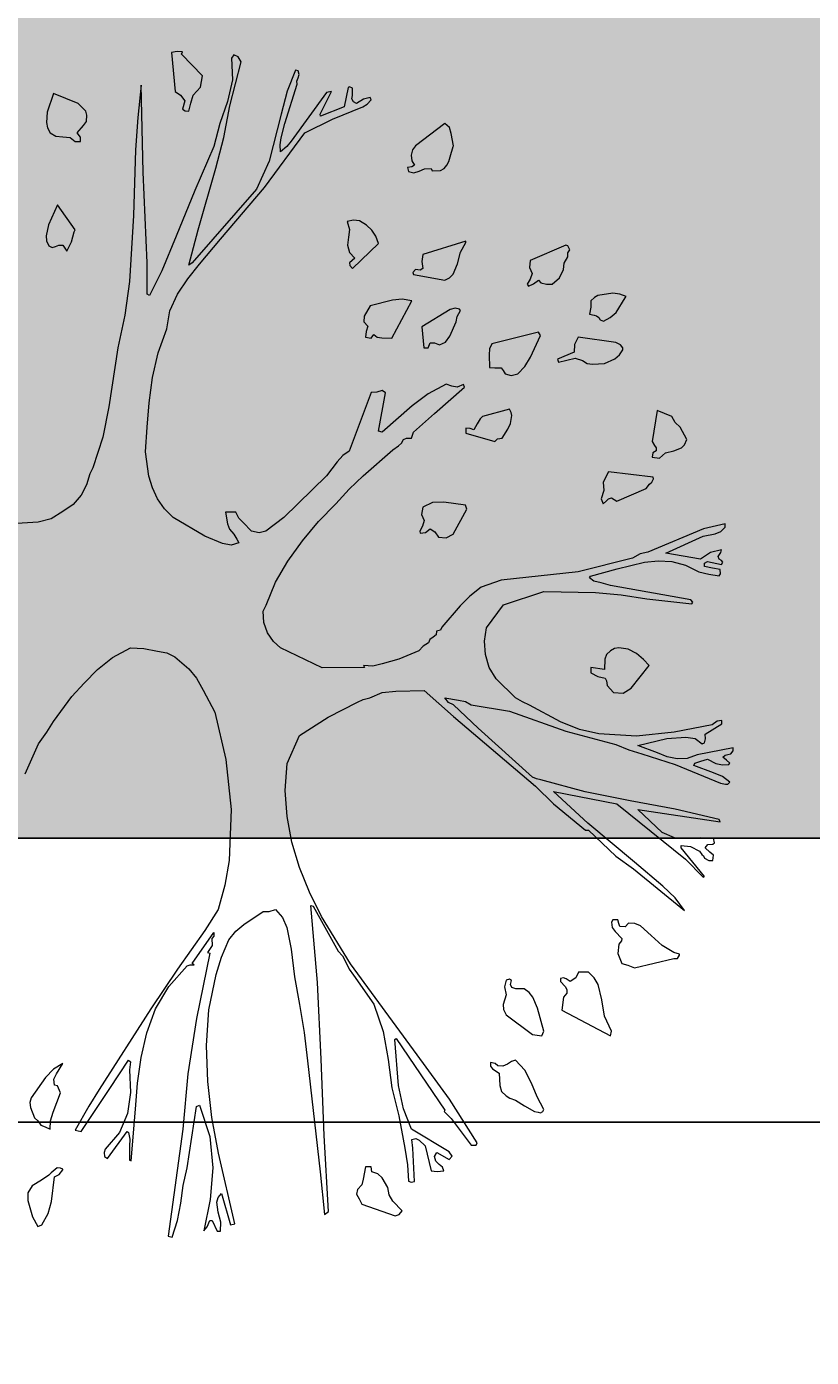
# Model space of a CAD drawing. Units: inches. Extents: x 84 to 1044, y -280 to 906.
# Tile 26 of 105: x 739 to 764, y -129 to -87. Entities that reach past the tile are written whole.
import ezdxf

# ---------------------------------------------------------------- set-up
doc = ezdxf.new("R2010")
doc.units = ezdxf.units.IN
for name, color, linetype, lineweight in [('A-ANNO-DIMS', 2, 'Continuous', 18), ('C-PROP', 7, 'Continuous', 25), ('L-PLNT', 114, 'Continuous', 15)]:
    doc.layers.add(name, color=color, linetype=linetype, lineweight=lineweight)
doc.layers.add('L-PLNT-PATT', color=9, linetype='Continuous', lineweight=9, true_color=0xafd9aa)
doc.styles.get("Standard").update_dxf_attribs({"font": 'arial.ttf'})
doc.dimstyles.get("Standard").update_dxf_attribs({"dimtxt": 0.18, "dimasz": 0.18, "dimexe": 0.18, "dimexo": 0.0625, "dimgap": 0.09, "dimtad": 0, "dimtih": 1, "dimtoh": 1, "dimdec": 4, "dimzin": 0, "dimdsep": 46, "dimtxsty": 'Standard', "dimcen": 0.09, "dimadec": 0, "dimazin": 0, "dimtfac": 1, "dimtdec": 4, "dimtofl": 0, "dimtmove": 0, "dimatfit": 3, "dimfxl": 1, "dimtolj": 1, "dimtzin": 0, "dimarcsym": 0})

# ---------------------------------------------------------------- blocks, each defined once
blk = doc.blocks.new('A$C37E508DF')
for p, q in [((0.7083, 1.5239), (0.7152, 1.5244)), ((0.7096, 1.5209), (0.7083, 1.5239)), ((0.7152, 1.5244), (0.7225, 1.5231)), ((0.7225, 1.5231), (0.7174, 1.4729)), ((0.6329, 1.5111), (0.6367, 1.5175)), ((0.6475, 1.4545), (0.6329, 1.5111)), ((0.6367, 1.5175), (0.6423, 1.5201)), ((0.6423, 1.5201), (0.6453, 1.5158)), ((0.6453, 1.5158), (0.644, 1.4879)), ((0.6826, 1.493), (0.7096, 1.5209)), ((0.5583, 1.4948), (0.5596, 1.4995)), ((0.5596, 1.4905), (0.5583, 1.4948)), ((0.5596, 1.4995), (0.563, 1.5003)), ((0.5613, 1.4862), (0.5596, 1.4905)), ((0.563, 1.5003), (0.5737, 1.4733)), ((0.6852, 1.4785), (0.6826, 1.493)), ((0.4897, 1.4772), (0.4935, 1.4789)), ((0.4897, 1.4678), (0.4897, 1.4772)), ((0.4935, 1.4789), (0.4952, 1.478)), ((0.4952, 1.478), (0.5004, 1.4532)), ((0.5313, 1.4437), (0.5167, 1.4729)), ((0.5167, 1.4729), (0.5231, 1.4716)), ((0.5231, 1.4716), (0.5686, 1.409)), ((0.5608, 1.4823), (0.5613, 1.4862)), ((0.5767, 1.4317), (0.5608, 1.4823)), ((0.5737, 1.4733), (0.5814, 1.4437)), ((0.644, 1.4879), (0.6505, 1.46)), ((0.6946, 1.4682), (0.6852, 1.4785)), ((0.7174, 1.4729), (0.7109, 1.4682)), ((0.7589, 1.3691), (0.7615, 1.481)), ((0.7615, 1.481), (0.7658, 1.4395)), ((0.4657, 1.4622), (0.4669, 1.4652)), ((0.4708, 1.4566), (0.4657, 1.4622)), ((0.4669, 1.4652), (0.4755, 1.463)), ((0.4764, 1.4532), (0.4708, 1.4566)), ((0.4755, 1.463), (0.4845, 1.4575)), ((0.4845, 1.4575), (0.4884, 1.4596)), ((0.4884, 1.4596), (0.4905, 1.4635)), ((0.4905, 1.4635), (0.4897, 1.4678)), ((0.6552, 1.4137), (0.6475, 1.4545)), ((0.6505, 1.46), (0.6603, 1.4317)), ((0.6976, 1.4579), (0.6946, 1.4682)), ((0.7002, 1.4476), (0.6976, 1.4579)), ((0.7109, 1.4682), (0.7053, 1.4609)), ((0.7053, 1.4609), (0.7083, 1.4502)), ((0.8357, 1.451), (0.8421, 1.4575)), ((0.8421, 1.4575), (0.8739, 1.4703)), ((0.8739, 1.4703), (0.882, 1.4463)), ((0.5154, 1.4373), (0.4764, 1.4532)), ((0.5004, 1.4532), (0.5308, 1.4412)), ((0.551, 1.4197), (0.5154, 1.4373)), ((0.5308, 1.4412), (0.5313, 1.4437)), ((0.5814, 1.4437), (0.5969, 1.3833)), ((0.7049, 1.448), (0.7002, 1.4476)), ((0.7083, 1.4502), (0.7049, 1.448)), ((0.7658, 1.4395), (0.7684, 1.3979)), ((0.831, 1.4424), (0.8323, 1.4476)), ((0.8318, 1.4343), (0.831, 1.4424)), ((0.8323, 1.4476), (0.8357, 1.451)), ((0.882, 1.4463), (0.8829, 1.433)), ((0.3628, 1.4189), (0.3649, 1.4266)), ((0.3649, 1.4266), (0.3709, 1.4317)), ((0.3709, 1.4317), (0.4086, 1.403)), ((0.5814, 1.4133), (0.5767, 1.4317)), ((0.6603, 1.4317), (0.668, 1.4021)), ((0.8353, 1.4292), (0.8318, 1.4343)), ((0.8434, 1.4197), (0.8353, 1.4292)), ((0.8816, 1.4262), (0.8781, 1.4197)), ((0.8829, 1.433), (0.8816, 1.4262)), ((0.3598, 1.403), (0.3628, 1.4189)), ((0.3602, 1.4021), (0.3598, 1.403)), ((0.4086, 1.403), (0.4125, 1.3979)), ((0.6029, 1.3494), (0.551, 1.4197)), ((0.5686, 1.409), (0.5741, 1.4021)), ((0.5827, 1.4043), (0.5814, 1.4133)), ((0.5823, 1.3953), (0.5827, 1.4043)), ((0.6655, 1.3743), (0.6552, 1.4137)), ((0.8391, 1.4141), (0.8434, 1.4197)), ((0.8395, 1.4086), (0.8391, 1.4141)), ((0.846, 1.4086), (0.8395, 1.4086)), ((0.8528, 1.4137), (0.846, 1.4086)), ((0.8619, 1.4146), (0.8528, 1.4137)), ((0.8709, 1.4154), (0.8619, 1.4146)), ((0.8781, 1.4197), (0.8709, 1.4154)), ((0.364, 1.3888), (0.3602, 1.4021)), ((0.3657, 1.3828), (0.364, 1.3888)), ((0.4125, 1.3979), (0.4142, 1.391)), ((0.4142, 1.391), (0.4134, 1.3837)), ((0.5741, 1.4021), (0.5823, 1.3953)), ((0.668, 1.4021), (0.6925, 1.3455)), ((0.7684, 1.3979), (0.771, 1.3134)), ((0.3683, 1.3781), (0.3657, 1.3828)), ((0.3718, 1.3738), (0.3683, 1.3781)), ((0.3765, 1.3713), (0.3718, 1.3738)), ((0.3872, 1.3708), (0.3765, 1.3713)), ((0.3885, 1.3738), (0.3872, 1.3708)), ((0.3971, 1.3734), (0.3885, 1.3738)), ((0.4039, 1.3704), (0.3971, 1.3734)), ((0.4108, 1.3683), (0.4039, 1.3704)), ((0.4134, 1.3837), (0.4099, 1.3781)), ((0.4099, 1.3781), (0.4134, 1.376)), ((0.4176, 1.37), (0.4108, 1.3683)), ((0.4134, 1.376), (0.4189, 1.3751)), ((0.4189, 1.3751), (0.4176, 1.37)), ((0.5969, 1.3833), (0.6132, 1.3472)), ((0.6882, 1.2949), (0.6655, 1.3743)), ((0.7538, 1.2529), (0.7589, 1.3691)), ((0.6595, 1.2829), (0.6029, 1.3494)), ((0.6132, 1.3472), (0.6959, 1.2529)), ((0.6925, 1.3455), (0.7161, 1.2868)), ((0.846, 1.2949), (0.8687, 1.3271)), ((0.8687, 1.3271), (0.8803, 1.3014)), ((0.4648, 1.2945), (0.4717, 1.3009)), ((0.4717, 1.3009), (0.4807, 1.3065)), ((0.4807, 1.3065), (0.4884, 1.3074)), ((0.4884, 1.3074), (0.4965, 1.3057)), ((0.4965, 1.3057), (0.4935, 1.2954)), ((0.771, 1.3134), (0.7761, 1.2285)), ((0.8803, 1.3014), (0.8833, 1.2872)), ((0.4562, 1.2774), (0.4597, 1.2868)), ((0.4597, 1.2868), (0.4648, 1.2945)), ((0.4935, 1.2954), (0.4948, 1.2855)), ((0.4948, 1.2855), (0.4961, 1.2756)), ((0.7002, 1.2495), (0.6882, 1.2949)), ((0.7161, 1.2868), (0.7349, 1.2422)), ((0.8473, 1.2924), (0.846, 1.2949)), ((0.8507, 1.2795), (0.8473, 1.2924)), ((0.8833, 1.2872), (0.8829, 1.2808)), ((0.2101, 1.2696), (0.2127, 1.2744)), ((0.2127, 1.2654), (0.2101, 1.2696)), ((0.2127, 1.2744), (0.2152, 1.2752)), ((0.2152, 1.2752), (0.2611, 1.2559)), ((0.3439, 1.2804), (0.3992, 1.2636)), ((0.3439, 1.2787), (0.3439, 1.2804)), ((0.3507, 1.2662), (0.3439, 1.2787)), ((0.3546, 1.2516), (0.3507, 1.2662)), ((0.4897, 1.2452), (0.4562, 1.2774)), ((0.4961, 1.2756), (0.4935, 1.2658)), ((0.6865, 1.2508), (0.6595, 1.2829)), ((0.8567, 1.2679), (0.8507, 1.2795)), ((0.8619, 1.2752), (0.8567, 1.2679)), ((0.867, 1.2752), (0.8619, 1.2752)), ((0.8713, 1.2739), (0.867, 1.2752)), ((0.8756, 1.2726), (0.8713, 1.2739)), ((0.8799, 1.2744), (0.8756, 1.2726)), ((0.8829, 1.2808), (0.8799, 1.2744)), ((0.2127, 1.2602), (0.2127, 1.2654)), ((0.2174, 1.2521), (0.2127, 1.2602)), ((0.2182, 1.2443), (0.2174, 1.2521)), ((0.2611, 1.2559), (0.262, 1.2465)), ((0.3602, 1.2383), (0.3546, 1.2516)), ((0.3992, 1.2636), (0.4005, 1.2546)), ((0.4005, 1.2546), (0.3992, 1.2452)), ((0.4935, 1.2658), (0.4867, 1.2589)), ((0.4867, 1.2589), (0.4935, 1.2529)), ((0.4931, 1.2491), (0.4897, 1.2452)), ((0.4935, 1.2529), (0.4931, 1.2491)), ((0.7015, 1.2323), (0.6865, 1.2508)), ((0.6959, 1.2529), (0.7002, 1.2495)), ((0.7538, 1.2122), (0.7538, 1.2529)), ((0.2234, 1.2336), (0.2182, 1.2443)), ((0.2328, 1.2251), (0.2234, 1.2336)), ((0.262, 1.2465), (0.2586, 1.2388)), ((0.2586, 1.2388), (0.2611, 1.2319)), ((0.2611, 1.2319), (0.265, 1.2251)), ((0.3649, 1.2336), (0.3602, 1.2383)), ((0.3709, 1.2306), (0.3649, 1.2336)), ((0.4112, 1.2375), (0.3709, 1.2306)), ((0.3992, 1.2452), (0.4026, 1.2431)), ((0.4026, 1.2431), (0.4086, 1.2443)), ((0.4086, 1.2443), (0.4121, 1.2401)), ((0.4121, 1.2401), (0.4112, 1.2375)), ((0.7148, 1.2126), (0.7015, 1.2323)), ((0.7349, 1.2422), (0.7482, 1.216)), ((0.2401, 1.2251), (0.2328, 1.2251)), ((0.2474, 1.2268), (0.2401, 1.2251)), ((0.2504, 1.2306), (0.2474, 1.2268)), ((0.2568, 1.2255), (0.2504, 1.2306)), ((0.2633, 1.2229), (0.2568, 1.2255)), ((0.265, 1.2251), (0.2633, 1.2229)), ((0.7482, 1.216), (0.7508, 1.2109)), ((0.7761, 1.2285), (0.7821, 1.1856)), ((0.1376, 1.2092), (0.1458, 1.2126)), ((0.1389, 1.2079), (0.1376, 1.2092)), ((0.1505, 1.189), (0.1389, 1.2079)), ((0.1458, 1.2126), (0.1548, 1.2135)), ((0.1548, 1.2135), (0.1741, 1.2109)), ((0.1741, 1.2109), (0.1784, 1.2083)), ((0.1784, 1.2083), (0.1831, 1.204)), ((0.1831, 1.204), (0.1831, 1.1959)), ((0.4134, 1.204), (0.4258, 1.2058)), ((0.4391, 1.156), (0.4134, 1.204)), ((0.4258, 1.2058), (0.4382, 1.2045)), ((0.4382, 1.2045), (0.4669, 1.1972)), ((0.7246, 1.1908), (0.7148, 1.2126)), ((0.7508, 1.2109), (0.7538, 1.2122)), ((0.1582, 1.1822), (0.1505, 1.189)), ((0.1668, 1.1775), (0.1582, 1.1822)), ((0.1728, 1.1826), (0.1711, 1.1792)), ((0.1758, 1.1847), (0.1728, 1.1826)), ((0.1788, 1.1852), (0.1758, 1.1847)), ((0.1848, 1.1865), (0.1788, 1.1852)), ((0.1831, 1.1959), (0.1848, 1.1865)), ((0.3507, 1.1916), (0.352, 1.1933)), ((0.355, 1.1839), (0.3507, 1.1916)), ((0.352, 1.1933), (0.3576, 1.1942)), ((0.3563, 1.177), (0.355, 1.1839)), ((0.3576, 1.1942), (0.364, 1.1929)), ((0.364, 1.1929), (0.4005, 1.1702)), ((0.4669, 1.1972), (0.4747, 1.1843)), ((0.4747, 1.1843), (0.4751, 1.177)), ((0.7281, 1.168), (0.7246, 1.1908)), ((0.7821, 1.1856), (0.7911, 1.1436)), ((0.1711, 1.1792), (0.1668, 1.1775)), ((0.2478, 1.1594), (0.2504, 1.1637)), ((0.2504, 1.1637), (0.3104, 1.1487)), ((0.3645, 1.1586), (0.3563, 1.177)), ((0.4005, 1.1702), (0.3979, 1.1436)), ((0.4751, 1.177), (0.47, 1.1714)), ((0.47, 1.1714), (0.4721, 1.1646)), ((0.4721, 1.1646), (0.473, 1.1573)), ((0.7396, 1.1371), (0.7281, 1.168)), ((0.1419, 1.1436), (0.1449, 1.1474)), ((0.1449, 1.1474), (0.1509, 1.1504)), ((0.1509, 1.1504), (0.1994, 1.1573)), ((0.1994, 1.1573), (0.2041, 1.1479)), ((0.2041, 1.1479), (0.2045, 1.138)), ((0.2607, 1.1316), (0.2478, 1.1594)), ((0.3104, 1.1487), (0.3134, 1.1423)), ((0.37, 1.1509), (0.3645, 1.1586)), ((0.3778, 1.1474), (0.37, 1.1509)), ((0.3842, 1.15), (0.3778, 1.1474)), ((0.3898, 1.15), (0.3842, 1.15)), ((0.3923, 1.1436), (0.3898, 1.15)), ((0.4519, 1.1564), (0.4391, 1.156)), ((0.458, 1.1573), (0.4519, 1.1564)), ((0.4622, 1.1607), (0.458, 1.1573)), ((0.4657, 1.156), (0.4622, 1.1607)), ((0.473, 1.1573), (0.4657, 1.156)), ((0.1419, 1.141), (0.1419, 1.1436)), ((0.1462, 1.1342), (0.1419, 1.141)), ((0.1522, 1.1294), (0.1462, 1.1342)), ((0.1655, 1.1234), (0.1522, 1.1294)), ((0.2032, 1.1303), (0.1938, 1.1273)), ((0.2247, 1.1251), (0.2032, 1.1303)), ((0.2045, 1.138), (0.226, 1.129)), ((0.268, 1.1196), (0.2607, 1.1316)), ((0.3134, 1.1423), (0.3139, 1.1346)), ((0.3139, 1.1346), (0.3134, 1.1183)), ((0.3979, 1.1436), (0.3923, 1.1436)), ((0.7469, 1.1054), (0.7396, 1.1371)), ((0.7911, 1.1436), (0.8027, 1.0677)), ((0.181, 1.1226), (0.1655, 1.1234)), ((0.1878, 1.1234), (0.181, 1.1226)), ((0.1938, 1.1273), (0.1878, 1.1234)), ((0.226, 1.129), (0.2247, 1.1251)), ((0.277, 1.1101), (0.268, 1.1196)), ((0.2959, 1.1144), (0.2933, 1.1101)), ((0.2984, 1.1179), (0.2959, 1.1144)), ((0.3066, 1.1179), (0.2984, 1.1179)), ((0.3134, 1.1183), (0.3066, 1.1179)), ((0.2856, 1.108), (0.277, 1.1101)), ((0.2933, 1.1101), (0.2856, 1.108)), ((0.3456, 1.093), (0.3469, 1.0964)), ((0.3469, 1.0964), (0.355, 1.093)), ((0.3619, 1.0943), (0.3692, 1.0968)), ((0.3692, 1.0968), (0.3923, 1.0844)), ((0.7512, 1.0728), (0.7469, 1.1054)), ((0.3842, 1.0591), (0.3456, 1.093)), ((0.355, 1.093), (0.3619, 1.0943)), ((0.3923, 1.0844), (0.4129, 1.069)), ((0.4472, 1.0857), (0.4515, 1.0887)), ((0.4562, 1.0364), (0.4472, 1.0857)), ((0.4515, 1.0887), (0.4584, 1.0865)), ((0.4584, 1.0865), (0.4657, 1.0861)), ((0.4657, 1.0861), (0.4939, 1.0107)), ((0.0789, 1.0552), (0.0978, 1.063)), ((0.0978, 1.063), (0.1042, 1.0231)), ((0.2856, 1.0604), (0.2877, 1.0647)), ((0.2877, 1.0647), (0.3224, 1.0552)), ((0.4129, 1.069), (0.4515, 1.0351)), ((0.7538, 1.0415), (0.7512, 1.0728)), ((0.8027, 1.0677), (0.8108, 1.0287)), ((0.0682, 1.0415), (0.0746, 1.0475)), ((0.0746, 1.0475), (0.0789, 1.0552)), ((0.2847, 1.0565), (0.2856, 1.0604)), ((0.2851, 1.054), (0.2847, 1.0565)), ((0.2864, 1.0463), (0.2851, 1.054)), ((0.2899, 1.039), (0.2864, 1.0463)), ((0.3224, 1.0552), (0.3255, 1.0522)), ((0.3255, 1.0522), (0.3293, 1.0458)), ((0.3293, 1.0458), (0.3336, 1.0381)), ((0.4112, 1.0351), (0.3842, 1.0591)), ((0.0596, 1.0257), (0.0682, 1.0415)), ((0.2972, 1.0274), (0.2899, 1.039)), ((0.3032, 1.0265), (0.2972, 1.0274)), ((0.3439, 1.0338), (0.3066, 1.0231)), ((0.3336, 1.0381), (0.3383, 1.0398)), ((0.3383, 1.0398), (0.3439, 1.0402)), ((0.3439, 1.0402), (0.3439, 1.0338)), ((0.4138, 1.0274), (0.4112, 1.0351)), ((0.4202, 1.0274), (0.4138, 1.0274)), ((0.4241, 1.0257), (0.4202, 1.0274)), ((0.4515, 1.0351), (0.4562, 1.0364)), ((0.7559, 1.0098), (0.7538, 1.0415)), ((0.8108, 1.0287), (0.8233, 0.9892)), ((0.0626, 1.0188), (0.0596, 1.0257)), ((0.0665, 1.0149), (0.0626, 1.0188)), ((0.0763, 1.0111), (0.0665, 1.0149)), ((0.087, 1.0085), (0.0763, 1.0111)), ((0.1012, 1.018), (0.099, 1.0149)), ((0.099, 1.0149), (0.099, 1.0111)), ((0.099, 1.0111), (0.1033, 1.0085)), ((0.1042, 1.0231), (0.1012, 1.018)), ((0.3066, 1.0231), (0.3032, 1.0265)), ((0.4267, 1.0209), (0.4241, 1.0257)), ((0.4305, 1.0175), (0.4267, 1.0209)), ((0.4378, 1.0124), (0.4305, 1.0175)), ((0.476, 0.9789), (0.4378, 1.0124)), ((0.4939, 1.0107), (0.5021, 1.0051)), ((0.7516, 0.9785), (0.7559, 1.0098)), ((0.0948, 1.0016), (0.087, 1.0085)), ((0.1042, 1.0029), (0.0948, 1.0016)), ((0.1033, 1.0085), (0.1042, 1.0029)), ((0.5021, 1.0051), (0.5094, 0.9969)), ((0.5094, 0.9969), (0.5231, 0.9789)), ((0.1025, 0.9751), (0.1029, 0.9772)), ((0.1029, 0.9772), (0.1604, 0.9841)), ((0.1604, 0.9841), (0.1672, 0.9708)), ((0.4939, 0.9618), (0.476, 0.9789)), ((0.5231, 0.9789), (0.578, 0.9253)), ((0.7469, 0.9635), (0.7516, 0.9785)), ((0.8233, 0.9892), (0.8275, 0.9815)), ((0.8275, 0.9815), (0.8314, 0.9673)), ((0.1046, 0.9708), (0.1025, 0.9751)), ((0.1076, 0.9682), (0.1046, 0.9708)), ((0.1119, 0.9626), (0.1076, 0.9682)), ((0.1496, 0.9463), (0.1119, 0.9626)), ((0.1672, 0.9708), (0.1664, 0.9601)), ((0.1664, 0.9601), (0.1698, 0.9493)), ((0.5111, 0.9429), (0.4939, 0.9618)), ((0.7401, 0.9493), (0.7469, 0.9635)), ((0.8314, 0.9673), (0.8383, 0.954)), ((0.1565, 0.9506), (0.1496, 0.9463)), ((0.1604, 0.9493), (0.1565, 0.9506)), ((0.1629, 0.9468), (0.1604, 0.9493)), ((0.1672, 0.9429), (0.1629, 0.9468)), ((0.1698, 0.9493), (0.1672, 0.9429)), ((0.3426, 0.936), (0.3443, 0.9412)), ((0.3443, 0.9412), (0.3722, 0.9451)), ((0.3722, 0.9451), (0.3868, 0.9446)), ((0.3868, 0.9446), (0.3992, 0.9386)), ((0.5334, 0.9202), (0.5111, 0.9429)), ((0.7315, 0.9365), (0.7401, 0.9493)), ((0.8383, 0.954), (0.8486, 0.942)), ((0.8486, 0.942), (0.8619, 0.933)), ((0.3602, 0.9039), (0.3426, 0.936)), ((0.4009, 0.9292), (0.3975, 0.9215)), ((0.3992, 0.9386), (0.4009, 0.9292)), ((0.578, 0.9253), (0.6011, 0.9077)), ((0.6303, 0.9189), (0.6359, 0.9245)), ((0.6359, 0.9245), (0.6397, 0.9322)), ((0.6397, 0.9322), (0.653, 0.9322)), ((0.653, 0.9322), (0.6505, 0.9172)), ((0.6796, 0.9013), (0.7203, 0.9253)), ((0.7203, 0.9253), (0.7315, 0.9365)), ((0.8619, 0.933), (0.8769, 0.9236)), ((0.0103, 0.9129), (0.0103, 0.9172)), ((0.0103, 0.9172), (0.0382, 0.9107)), ((0.0159, 0.9073), (0.0103, 0.9129)), ((0.0232, 0.9043), (0.0159, 0.9073)), ((0.0382, 0.9107), (0.1098, 0.8807)), ((0.3838, 0.9069), (0.379, 0.9)), ((0.3898, 0.9107), (0.3838, 0.9069)), ((0.3958, 0.906), (0.3898, 0.9107)), ((0.3975, 0.9215), (0.3996, 0.9142)), ((0.3996, 0.9142), (0.4031, 0.9077)), ((0.4031, 0.9077), (0.4026, 0.9052)), ((0.554, 0.8953), (0.5334, 0.9202)), ((0.6011, 0.9077), (0.6097, 0.9056)), ((0.6097, 0.9056), (0.6196, 0.9077)), ((0.6196, 0.9077), (0.6303, 0.9189)), ((0.6479, 0.9103), (0.6423, 0.9039)), ((0.6505, 0.9172), (0.6479, 0.9103)), ((0.8769, 0.9236), (0.8936, 0.9193)), ((0.8936, 0.9193), (0.9279, 0.9172)), ((0.0386, 0.9013), (0.0232, 0.9043)), ((0.0866, 0.8794), (0.0386, 0.9013)), ((0.3692, 0.8992), (0.3602, 0.9039)), ((0.379, 0.9), (0.3692, 0.8992)), ((0.4026, 0.9052), (0.3958, 0.906)), ((0.5728, 0.8691), (0.554, 0.8953)), ((0.6384, 0.8974), (0.6359, 0.8927)), ((0.6359, 0.8927), (0.6457, 0.8897)), ((0.6423, 0.9039), (0.6384, 0.8974)), ((0.6457, 0.8897), (0.6569, 0.8919)), ((0.6569, 0.8919), (0.6796, 0.9013)), ((0.0159, 0.8803), (0.0154, 0.8837)), ((0.0154, 0.8837), (0.0292, 0.8803)), ((0.0176, 0.8777), (0.0159, 0.8803)), ((0.0193, 0.8752), (0.0176, 0.8777)), ((0.0184, 0.8717), (0.0193, 0.8752)), ((0.0292, 0.8803), (0.0424, 0.8717)), ((0.0424, 0.8717), (0.0866, 0.8794)), ((0.1098, 0.8807), (0.1196, 0.8786)), ((0.1196, 0.8786), (0.1295, 0.873)), ((0.1295, 0.873), (0.1994, 0.8554)), ((0.0133, 0.8679), (0.015, 0.87)), ((0.0154, 0.8649), (0.0133, 0.8679)), ((0.015, 0.87), (0.0184, 0.8717)), ((0.0334, 0.8687), (0.0154, 0.8649)), ((0.0163, 0.8529), (0.0171, 0.8584)), ((0.0171, 0.8584), (0.0266, 0.8602)), ((0.0266, 0.8602), (0.0369, 0.8623)), ((0.0369, 0.8666), (0.0334, 0.8687)), ((0.0369, 0.8623), (0.0369, 0.8666)), ((0.0617, 0.864), (0.0442, 0.8554)), ((0.0789, 0.8687), (0.0617, 0.864)), ((0.0965, 0.8696), (0.0789, 0.8687)), ((0.1141, 0.8679), (0.0965, 0.8696)), ((0.1492, 0.8593), (0.1141, 0.8679)), ((0.1835, 0.8499), (0.1492, 0.8593)), ((0.5887, 0.8421), (0.5728, 0.8691)), ((0.0184, 0.8503), (0.0163, 0.8529)), ((0.0317, 0.8524), (0.0184, 0.8503)), ((0.0442, 0.8554), (0.0317, 0.8524)), ((0.1578, 0.8378), (0.1698, 0.8413)), ((0.1698, 0.8413), (0.1792, 0.8434)), ((0.1792, 0.8434), (0.1848, 0.8477)), ((0.1848, 0.8477), (0.1835, 0.8499)), ((0.1994, 0.8554), (0.2984, 0.8447)), ((0.2984, 0.8447), (0.3242, 0.8357)), ((0.6007, 0.8125), (0.5887, 0.8421)), ((0.0545, 0.8194), (0.1578, 0.8378)), ((0.1441, 0.8258), (0.1111, 0.8207)), ((0.1771, 0.8288), (0.1441, 0.8258)), ((0.2436, 0.8301), (0.1771, 0.8288)), ((0.2954, 0.813), (0.2436, 0.8301)), ((0.3242, 0.8357), (0.3387, 0.8241)), ((0.3387, 0.8241), (0.3512, 0.8117)), ((0.0519, 0.8164), (0.0545, 0.8194)), ((0.0532, 0.8143), (0.0519, 0.8164)), ((0.1111, 0.8207), (0.0532, 0.8143)), ((0.3173, 0.7834), (0.2954, 0.813)), ((0.3512, 0.8117), (0.3748, 0.7842)), ((0.6046, 0.8048), (0.6007, 0.8125)), ((0.6037, 0.7903), (0.6046, 0.8048)), ((0.599, 0.777), (0.6037, 0.7903)), ((0.3199, 0.7662), (0.3173, 0.7834)), ((0.3748, 0.7842), (0.3765, 0.7804)), ((0.3765, 0.7804), (0.3816, 0.7791)), ((0.3816, 0.7791), (0.382, 0.7744)), ((0.382, 0.7744), (0.3859, 0.7714)), ((0.3859, 0.7714), (0.3902, 0.7684)), ((0.5913, 0.7658), (0.599, 0.777)), ((0.1244, 0.7504), (0.1351, 0.7559)), ((0.1351, 0.7559), (0.1471, 0.7577)), ((0.1471, 0.7577), (0.1527, 0.7568)), ((0.1527, 0.7568), (0.1578, 0.7538)), ((0.1578, 0.7538), (0.1629, 0.7491)), ((0.3186, 0.7491), (0.3199, 0.7662)), ((0.3902, 0.7684), (0.3919, 0.7641)), ((0.3919, 0.7641), (0.3988, 0.7598)), ((0.3988, 0.7598), (0.4043, 0.7538)), ((0.4043, 0.7538), (0.4301, 0.7431)), ((0.5287, 0.7319), (0.5823, 0.7577)), ((0.5823, 0.7577), (0.5913, 0.7658)), ((0.7401, 0.7534), (0.7285, 0.7512)), ((0.7577, 0.7568), (0.7401, 0.7534)), ((0.7752, 0.7577), (0.7577, 0.7568)), ((0.798, 0.7452), (0.7752, 0.7577)), ((0.1081, 0.7349), (0.1153, 0.7427)), ((0.1153, 0.7427), (0.1244, 0.7504)), ((0.1629, 0.7491), (0.1651, 0.7431)), ((0.1651, 0.7431), (0.1655, 0.7298)), ((0.3139, 0.7324), (0.3186, 0.7491)), ((0.4301, 0.7431), (0.4515, 0.7371)), ((0.4515, 0.7371), (0.4635, 0.7341)), ((0.7182, 0.7461), (0.7002, 0.7307)), ((0.7285, 0.7512), (0.7182, 0.7461)), ((0.8173, 0.7298), (0.798, 0.7452)), ((0.1312, 0.7058), (0.1081, 0.7349)), ((0.1646, 0.7186), (0.1629, 0.7152)), ((0.1741, 0.7208), (0.1646, 0.7186)), ((0.1655, 0.7298), (0.1831, 0.7324)), ((0.1831, 0.7255), (0.1741, 0.7208)), ((0.1831, 0.7324), (0.1831, 0.7255)), ((0.3049, 0.7178), (0.3139, 0.7324)), ((0.4635, 0.7341), (0.4755, 0.7349)), ((0.4755, 0.7349), (0.4742, 0.7324)), ((0.4742, 0.7324), (0.5287, 0.7319)), ((0.6903, 0.7186), (0.6818, 0.7032)), ((0.7002, 0.7307), (0.6903, 0.7186)), ((0.8344, 0.7122), (0.8173, 0.7298)), ((0.1415, 0.6994), (0.1312, 0.7058)), ((0.1621, 0.7092), (0.1539, 0.7002)), ((0.1629, 0.7152), (0.1621, 0.7092)), ((0.28, 0.6933), (0.3049, 0.7178)), ((0.3975, 0.7028), (0.3598, 0.6693)), ((0.4339, 0.7019), (0.3975, 0.7028)), ((0.4515, 0.7002), (0.4339, 0.7019)), ((0.6818, 0.7032), (0.6667, 0.6749)), ((0.8503, 0.6951), (0.8344, 0.7122)), ((0.1539, 0.7002), (0.1415, 0.6994)), ((0.262, 0.6839), (0.271, 0.6882)), ((0.271, 0.6882), (0.28, 0.6933)), ((0.3443, 0.6886), (0.337, 0.6843)), ((0.3533, 0.6903), (0.3443, 0.6886)), ((0.3709, 0.6933), (0.3533, 0.6903)), ((0.3598, 0.6843), (0.3662, 0.6873)), ((0.3662, 0.6873), (0.3709, 0.6933)), ((0.4674, 0.6933), (0.4515, 0.7002)), ((0.476, 0.6912), (0.4674, 0.6933)), ((0.4832, 0.6878), (0.476, 0.6912)), ((0.521, 0.6685), (0.4832, 0.6878)), ((0.8739, 0.6629), (0.8503, 0.6951)), ((0.2877, 0.6762), (0.2152, 0.6505)), ((0.2221, 0.6625), (0.262, 0.6839)), ((0.3598, 0.6693), (0.2543, 0.5797)), ((0.337, 0.6843), (0.2877, 0.6762)), ((0.328, 0.6543), (0.3598, 0.6843)), ((0.5578, 0.6449), (0.521, 0.6685)), ((0.6667, 0.6749), (0.6526, 0.614)), ((0.0146, 0.6599), (0.0146, 0.6642)), ((0.0146, 0.6642), (0.0206, 0.6633)), ((0.036, 0.6466), (0.0146, 0.6599)), ((0.0206, 0.6633), (0.0274, 0.6586)), ((0.0274, 0.6586), (0.0759, 0.6492)), ((0.2152, 0.6505), (0.1509, 0.6333)), ((0.1728, 0.647), (0.1977, 0.6526)), ((0.1977, 0.6526), (0.2221, 0.6625)), ((0.2581, 0.5913), (0.328, 0.6543)), ((0.8824, 0.6492), (0.8739, 0.6629)), ((0.0356, 0.6406), (0.036, 0.6466)), ((0.0369, 0.6355), (0.0356, 0.6406)), ((0.0399, 0.6342), (0.0369, 0.6355)), ((0.0489, 0.641), (0.0399, 0.6342)), ((0.0609, 0.6428), (0.0489, 0.641)), ((0.0853, 0.641), (0.0609, 0.6428)), ((0.0759, 0.6492), (0.1244, 0.644)), ((0.1226, 0.632), (0.0853, 0.641)), ((0.1244, 0.644), (0.1728, 0.647)), ((0.1509, 0.6333), (0.1342, 0.6265)), ((0.5737, 0.6089), (0.5578, 0.6449)), ((0.8932, 0.6342), (0.8824, 0.6492)), ((0.9103, 0.5956), (0.8932, 0.6342)), ((0, 0.629), (0.0467, 0.62)), ((0, 0.6252), (0, 0.629)), ((0.003, 0.6213), (0, 0.6252)), ((0.0069, 0.6204), (0.003, 0.6213)), ((0.0107, 0.6196), (0.0069, 0.6204)), ((0.0086, 0.6132), (0.0133, 0.617)), ((0.0133, 0.617), (0.0107, 0.6196)), ((0.0467, 0.62), (0.0592, 0.6153)), ((0.072, 0.6149), (0.0849, 0.6175)), ((0.1175, 0.6213), (0.0746, 0.6076)), ((0.0849, 0.6175), (0.0973, 0.6226)), ((0.0973, 0.6226), (0.1226, 0.632)), ((0.1342, 0.6265), (0.1175, 0.6213)), ((0.0047, 0.6093), (0.0086, 0.6132)), ((0.0056, 0.6076), (0.0047, 0.6093)), ((0.0141, 0.6072), (0.0056, 0.6076)), ((0.0223, 0.6089), (0.0141, 0.6072)), ((0.0746, 0.6076), (0.0163, 0.5836)), ((0.0334, 0.6145), (0.0223, 0.6089)), ((0.0257, 0.5969), (0.0506, 0.6063)), ((0.0416, 0.6119), (0.0334, 0.6145)), ((0.0493, 0.6093), (0.0416, 0.6119)), ((0.0506, 0.6063), (0.0493, 0.6093)), ((0.0592, 0.6153), (0.072, 0.6149)), ((0.5763, 0.5741), (0.5737, 0.6089)), ((0.6526, 0.614), (0.6457, 0.5497)), ((0.0047, 0.5849), (0.0141, 0.5921)), ((0.0069, 0.5823), (0.0047, 0.5849)), ((0.0099, 0.5823), (0.0069, 0.5823)), ((0.0163, 0.5836), (0.0099, 0.5823)), ((0.0141, 0.5921), (0.0257, 0.5969)), ((0.1904, 0.5724), (0.2474, 0.5879)), ((0.2474, 0.5879), (0.253, 0.5892)), ((0.253, 0.5892), (0.2581, 0.5913)), ((0.1325, 0.5608), (0.1904, 0.5724)), ((0.2311, 0.5729), (0.1496, 0.557)), ((0.1869, 0.5325), (0.2311, 0.5729)), ((0.2543, 0.5797), (0.2311, 0.557)), ((0.5737, 0.5407), (0.5763, 0.5741)), ((0.1226, 0.5497), (0.0171, 0.5338)), ((0.0184, 0.5368), (0.0746, 0.5501)), ((0.1496, 0.557), (0.0613, 0.4858)), ((0.0746, 0.5501), (0.1325, 0.5608)), ((0.0917, 0.5205), (0.1226, 0.5497)), ((0.2311, 0.557), (0.1899, 0.5235)), ((0.6457, 0.5497), (0.6483, 0.4845)), ((0.0171, 0.5338), (0.0184, 0.5368)), ((0.1269, 0.482), (0.1869, 0.5325)), ((0.5677, 0.5077), (0.5737, 0.5407)), ((0.0755, 0.5133), (0.0917, 0.5205)), ((0.1861, 0.5231), (0.1509, 0.4897)), ((0.1899, 0.5235), (0.1861, 0.5231)), ((0.024, 0.5072), (0.0253, 0.5128)), ((0.0262, 0.5055), (0.024, 0.5072)), ((0.0253, 0.5128), (0.042, 0.5133)), ((0.0326, 0.5047), (0.0262, 0.5055)), ((0.03, 0.4948), (0.036, 0.5004)), ((0.036, 0.5004), (0.0326, 0.5047)), ((0.0369, 0.4639), (0.0669, 0.5004)), ((0.042, 0.5133), (0.0587, 0.5124)), ((0.0549, 0.5021), (0.0437, 0.4961)), ((0.0669, 0.5034), (0.0549, 0.5021)), ((0.0587, 0.5124), (0.0755, 0.5133)), ((0.0669, 0.5004), (0.0669, 0.5034)), ((0.5578, 0.4751), (0.5677, 0.5077)), ((0.0253, 0.491), (0.03, 0.4948)), ((0.0262, 0.4841), (0.0253, 0.491)), ((0.0317, 0.4841), (0.0262, 0.4841)), ((0.0369, 0.4871), (0.0317, 0.4841)), ((0.0382, 0.4905), (0.0369, 0.4871)), ((0.0403, 0.4922), (0.0382, 0.4905)), ((0.0613, 0.4858), (0.0386, 0.4627)), ((0.0437, 0.4961), (0.0403, 0.4922)), ((0.0905, 0.4515), (0.1269, 0.482)), ((0.1509, 0.4897), (0.1282, 0.4734)), ((0.6483, 0.4845), (0.6539, 0.4524)), ((0.0386, 0.4627), (0.0369, 0.4639)), ((0.1282, 0.4734), (0.0626, 0.4198)), ((0.545, 0.4434), (0.5578, 0.4751)), ((0.0746, 0.4361), (0.0905, 0.4515)), ((0.6539, 0.4524), (0.6625, 0.4211)), ((0.0626, 0.4198), (0.0746, 0.4361)), ((0.5295, 0.4125), (0.545, 0.4434)), ((0.4922, 0.3516), (0.5295, 0.4125)), ((0.5403, 0.4254), (0.5081, 0.3679)), ((0.5347, 0.3276), (0.5433, 0.4266)), ((0.5433, 0.4266), (0.5403, 0.4254)), ((0.5797, 0.4112), (0.5741, 0.3983)), ((0.5887, 0.4215), (0.5797, 0.4112)), ((0.5969, 0.4189), (0.5887, 0.4215)), ((0.6046, 0.4189), (0.5969, 0.4189)), ((0.6295, 0.4022), (0.6046, 0.4189)), ((0.6625, 0.4211), (0.6796, 0.3945)), ((0.1055, 0.388), (0.1192, 0.4001)), ((0.1192, 0.4001), (0.1265, 0.4031)), ((0.1265, 0.4031), (0.1346, 0.4039)), ((0.1346, 0.4039), (0.1389, 0.3992)), ((0.1389, 0.3992), (0.1458, 0.3996)), ((0.1458, 0.3996), (0.1471, 0.4035)), ((0.1471, 0.4035), (0.1484, 0.4082)), ((0.1484, 0.4082), (0.1548, 0.4082)), ((0.1556, 0.3983), (0.1518, 0.3932)), ((0.1548, 0.4082), (0.1565, 0.4052)), ((0.1565, 0.4052), (0.1556, 0.3983)), ((0.5741, 0.3983), (0.5686, 0.3705)), ((0.6397, 0.3936), (0.6295, 0.4022)), ((0.6487, 0.3825), (0.6397, 0.3936)), ((0.6796, 0.3945), (0.7148, 0.3447)), ((0.0917, 0.3748), (0.1055, 0.388)), ((0.1518, 0.3932), (0.1432, 0.3842)), ((0.1432, 0.3842), (0.1436, 0.3808)), ((0.1436, 0.3808), (0.1471, 0.3769)), ((0.1471, 0.3769), (0.1484, 0.3649)), ((0.6582, 0.3602), (0.6487, 0.3825)), ((0.6959, 0.352), (0.668, 0.3919)), ((0.668, 0.3919), (0.668, 0.3872)), ((0.668, 0.3872), (0.6706, 0.3842)), ((0.6706, 0.3842), (0.6702, 0.3748)), ((0.069, 0.364), (0.0763, 0.3662)), ((0.069, 0.3627), (0.069, 0.364)), ((0.0716, 0.3585), (0.069, 0.3627)), ((0.0763, 0.3662), (0.0917, 0.3748)), ((0.1484, 0.3649), (0.1432, 0.352)), ((0.5025, 0.3619), (0.4982, 0.3537)), ((0.5081, 0.3679), (0.5025, 0.3619)), ((0.5686, 0.3705), (0.5643, 0.3349)), ((0.665, 0.3379), (0.6582, 0.3602)), ((0.6702, 0.3748), (0.6762, 0.3662)), ((0.6762, 0.3662), (0.6732, 0.3653)), ((0.6732, 0.3653), (0.6903, 0.2813)), ((0.0763, 0.3585), (0.0716, 0.3585)), ((0.1269, 0.3464), (0.0763, 0.3585)), ((0.1355, 0.3499), (0.1269, 0.3464)), ((0.1432, 0.352), (0.1355, 0.3499)), ((0.4065, 0.2345), (0.4922, 0.3516)), ((0.4939, 0.3447), (0.4884, 0.337)), ((0.4982, 0.3537), (0.4939, 0.3447)), ((0.6933, 0.3503), (0.6959, 0.352)), ((0.6985, 0.3503), (0.6933, 0.3503)), ((0.7023, 0.349), (0.6985, 0.3503)), ((0.7259, 0.3224), (0.7023, 0.349)), ((0.7148, 0.3447), (0.7487, 0.2937)), ((0.1737, 0.325), (0.1788, 0.3336)), ((0.1788, 0.3336), (0.1861, 0.3409)), ((0.1861, 0.3409), (0.199, 0.3409)), ((0.199, 0.3409), (0.2024, 0.3336)), ((0.2024, 0.3336), (0.2097, 0.3289)), ((0.2097, 0.3289), (0.2148, 0.3323)), ((0.2148, 0.3323), (0.2182, 0.3336)), ((0.2221, 0.3289), (0.2161, 0.3224)), ((0.2182, 0.3336), (0.2221, 0.3327)), ((0.2221, 0.3327), (0.2221, 0.3289)), ((0.2851, 0.3302), (0.2877, 0.3319)), ((0.2864, 0.325), (0.2851, 0.3302)), ((0.2877, 0.3319), (0.292, 0.3306)), ((0.292, 0.3306), (0.2941, 0.322)), ((0.4884, 0.337), (0.4622, 0.2997)), ((0.53, 0.229), (0.5347, 0.3276)), ((0.5643, 0.3349), (0.5578, 0.2993)), ((0.6745, 0.2924), (0.665, 0.3379)), ((0.1689, 0.3053), (0.1737, 0.325)), ((0.2161, 0.3224), (0.214, 0.3186)), ((0.214, 0.3186), (0.214, 0.3139)), ((0.214, 0.3139), (0.2182, 0.3087)), ((0.2182, 0.3087), (0.2204, 0.292)), ((0.2517, 0.2946), (0.2577, 0.3087)), ((0.2577, 0.3087), (0.2624, 0.3147)), ((0.2624, 0.3147), (0.2689, 0.3194)), ((0.2689, 0.3194), (0.2796, 0.3194)), ((0.2796, 0.3194), (0.2847, 0.3211)), ((0.2847, 0.3211), (0.2864, 0.325)), ((0.2941, 0.322), (0.292, 0.3117)), ((0.292, 0.3117), (0.2959, 0.2993)), ((0.7427, 0.2937), (0.7259, 0.3224)), ((0.2204, 0.292), (0.1578, 0.259)), ((0.1655, 0.2843), (0.1689, 0.3053)), ((0.2436, 0.265), (0.2517, 0.2946)), ((0.2954, 0.2928), (0.292, 0.286)), ((0.2959, 0.2993), (0.2954, 0.2928)), ((0.4622, 0.2997), (0.4502, 0.2645)), ((0.5578, 0.2993), (0.5518, 0.2633)), ((0.6775, 0.2465), (0.6745, 0.2924)), ((0.7542, 0.2628), (0.7427, 0.2937)), ((0.7487, 0.2937), (0.8151, 0.1899)), ((0.1565, 0.265), (0.1655, 0.2843)), ((0.292, 0.286), (0.2581, 0.2607)), ((0.6903, 0.2813), (0.7015, 0.2101)), ((0.1578, 0.259), (0.1565, 0.265)), ((0.2461, 0.259), (0.2436, 0.265)), ((0.2581, 0.2607), (0.2461, 0.259)), ((0.4502, 0.2645), (0.4438, 0.2285)), ((0.5518, 0.2633), (0.5475, 0.2268)), ((0.7615, 0.2311), (0.7542, 0.2628)), ((0.4335, 0.2556), (0.3709, 0.1634)), ((0.4305, 0.1951), (0.4352, 0.2543)), ((0.4352, 0.2543), (0.4335, 0.2556)), ((0.6758, 0.2002), (0.6775, 0.2465)), ((0.268, 0.2148), (0.28, 0.2277)), ((0.28, 0.2277), (0.2851, 0.226)), ((0.2851, 0.226), (0.2903, 0.2225)), ((0.2903, 0.2225), (0.2963, 0.22)), ((0.3027, 0.2204), (0.3061, 0.2234)), ((0.3061, 0.2234), (0.3122, 0.2247)), ((0.3122, 0.2247), (0.3122, 0.22)), ((0.3649, 0.1775), (0.4065, 0.2345)), ((0.4438, 0.2285), (0.4391, 0.1921)), ((0.5261, 0.1308), (0.53, 0.229)), ((0.5475, 0.2268), (0.5313, 0.084)), ((0.7662, 0.1981), (0.7615, 0.2311)), ((0.7778, 0.2277), (0.7752, 0.2255)), ((0.7752, 0.2255), (0.7761, 0.2152)), ((0.8018, 0.1912), (0.7778, 0.2277)), ((0.8619, 0.2234), (0.8739, 0.2161)), ((0.87, 0.2101), (0.8619, 0.2234)), ((0.2594, 0.1981), (0.268, 0.2148)), ((0.2963, 0.22), (0.3027, 0.2204)), ((0.301, 0.211), (0.3002, 0.1951)), ((0.3096, 0.2165), (0.301, 0.211)), ((0.3122, 0.22), (0.3096, 0.2165)), ((0.7015, 0.2101), (0.7079, 0.1389)), ((0.7761, 0.2152), (0.7752, 0.1861)), ((0.8734, 0.2032), (0.87, 0.2101)), ((0.8739, 0.2161), (0.8841, 0.2054)), ((0.8841, 0.2054), (0.9026, 0.1792)), ((0.2521, 0.1805), (0.2594, 0.1981)), ((0.3002, 0.1951), (0.298, 0.1874)), ((0.4241, 0.1651), (0.4305, 0.1951)), ((0.4391, 0.1921), (0.4301, 0.1561)), ((0.6706, 0.1539), (0.6758, 0.2002)), ((0.7688, 0.1646), (0.7662, 0.1981)), ((0.8383, 0.1359), (0.8018, 0.1912)), ((0.8151, 0.1899), (0.8288, 0.1685)), ((0.8649, 0.1857), (0.8687, 0.1947)), ((0.8687, 0.1947), (0.8726, 0.1955)), ((0.8726, 0.1955), (0.8734, 0.2032)), ((0.2436, 0.1642), (0.2521, 0.1805)), ((0.28, 0.1762), (0.2684, 0.1689)), ((0.2873, 0.1788), (0.28, 0.1762)), ((0.292, 0.1818), (0.2873, 0.1788)), ((0.298, 0.1874), (0.292, 0.1818)), ((0.3293, 0.1213), (0.3649, 0.1775)), ((0.7752, 0.1861), (0.7787, 0.1591)), ((0.8743, 0.1608), (0.8649, 0.1857)), ((0.9026, 0.1792), (0.9043, 0.1732)), ((0.9043, 0.1732), (0.9035, 0.1668)), ((0.2448, 0.1616), (0.2436, 0.1642)), ((0.2478, 0.1599), (0.2448, 0.1616)), ((0.2508, 0.1608), (0.2478, 0.1599)), ((0.2556, 0.1616), (0.2508, 0.1608)), ((0.2684, 0.1689), (0.2556, 0.1616)), ((0.3692, 0.1591), (0.3628, 0.1526)), ((0.3718, 0.1616), (0.3692, 0.1591)), ((0.3709, 0.1634), (0.3718, 0.1616)), ((0.4138, 0.1389), (0.4241, 0.1651)), ((0.4301, 0.1561), (0.4224, 0.1145)), ((0.6865, 0.1698), (0.6732, 0.1295)), ((0.6903, 0.1681), (0.6865, 0.1698)), ((0.7023, 0.0892), (0.6903, 0.1681)), ((0.774, 0.0982), (0.7688, 0.1646)), ((0.7787, 0.1591), (0.789, 0.1346)), ((0.8288, 0.1685), (0.846, 0.1376)), ((0.8777, 0.1496), (0.8743, 0.1608)), ((0.9035, 0.1668), (0.8983, 0.1535)), ((0.3628, 0.1526), (0.337, 0.1183)), ((0.3653, 0.1098), (0.4138, 0.1389)), ((0.662, 0.108), (0.6706, 0.1539)), ((0.7079, 0.1389), (0.7268, 0.0013)), ((0.846, 0.1376), (0.8383, 0.1359)), ((0.8781, 0.1389), (0.8777, 0.1496)), ((0.8846, 0.1419), (0.8781, 0.1389)), ((0.8902, 0.1441), (0.8846, 0.1419)), ((0.894, 0.1496), (0.8902, 0.1441)), ((0.8983, 0.1535), (0.894, 0.1496)), ((0.3306, 0.1183), (0.3293, 0.1213)), ((0.4039, 0.1248), (0.3962, 0.1175)), ((0.4082, 0.1269), (0.4039, 0.1248)), ((0.4134, 0.1256), (0.4082, 0.1269)), ((0.4121, 0.1145), (0.4134, 0.1256)), ((0.5205, 0.033), (0.5261, 0.1308)), ((0.6732, 0.1295), (0.6693, 0.0892)), ((0.7774, 0.1346), (0.7757, 0.1261)), ((0.7757, 0.1261), (0.7761, 0.117)), ((0.7791, 0.1359), (0.7774, 0.1346)), ((0.8044, 0.1012), (0.7791, 0.1359)), ((0.789, 0.1346), (0.8074, 0.1132)), ((0.337, 0.1183), (0.3306, 0.1183)), ((0.3615, 0.1042), (0.3653, 0.1098)), ((0.3653, 0.0999), (0.3615, 0.1042)), ((0.3812, 0.1089), (0.3653, 0.0999)), ((0.3842, 0.1037), (0.3812, 0.1089)), ((0.3825, 0.0978), (0.3842, 0.1037)), ((0.3962, 0.1175), (0.3885, 0.0853)), ((0.4099, 0.0716), (0.4121, 0.1145)), ((0.4224, 0.1145), (0.4189, 0.093)), ((0.641, 0.0172), (0.662, 0.108)), ((0.7761, 0.117), (0.7761, 0.099)), ((0.8083, 0.1037), (0.8044, 0.1012)), ((0.8074, 0.1132), (0.8087, 0.1089)), ((0.8087, 0.1089), (0.8083, 0.1037)), ((0.3722, 0.0853), (0.3739, 0.09)), ((0.3739, 0.09), (0.3782, 0.0935)), ((0.3782, 0.0935), (0.3825, 0.0978)), ((0.4189, 0.093), (0.4176, 0.072)), ((0.4648, 0.084), (0.4657, 0.0905)), ((0.4657, 0.0905), (0.473, 0.0905)), ((0.473, 0.0905), (0.476, 0.0746)), ((0.6693, 0.0892), (0.6728, 0.0484)), ((0.7075, 0.0665), (0.7023, 0.0892)), ((0.7761, 0.099), (0.774, 0.0982)), ((0.8619, 0.0875), (0.8649, 0.0887)), ((0.8619, 0.0866), (0.8619, 0.0875)), ((0.8666, 0.0806), (0.8619, 0.0866)), ((0.8649, 0.0887), (0.8691, 0.0892)), ((0.8691, 0.0892), (0.8769, 0.0827)), ((0.3808, 0.0845), (0.3722, 0.0853)), ((0.3885, 0.0853), (0.3808, 0.0845)), ((0.4142, 0.0707), (0.4099, 0.0716)), ((0.4176, 0.072), (0.4142, 0.0707)), ((0.4442, 0.0639), (0.4515, 0.0763)), ((0.4515, 0.0763), (0.4571, 0.0815)), ((0.4571, 0.0815), (0.4648, 0.084)), ((0.476, 0.0746), (0.4777, 0.0673)), ((0.5313, 0.084), (0.5257, 0.0291)), ((0.8726, 0.0776), (0.8666, 0.0806)), ((0.8764, 0.0459), (0.8726, 0.0776)), ((0.8769, 0.0827), (0.8799, 0.0797)), ((0.8799, 0.0797), (0.8893, 0.0733)), ((0.8893, 0.0733), (0.9013, 0.066)), ((0.4378, 0.0463), (0.4425, 0.0544)), ((0.4425, 0.0544), (0.4442, 0.0639)), ((0.4777, 0.0673), (0.4832, 0.0613)), ((0.4845, 0.0553), (0.4811, 0.0493)), ((0.4832, 0.0613), (0.4845, 0.0553)), ((0.6582, 0.0562), (0.6466, 0.0159)), ((0.6625, 0.051), (0.6582, 0.0562)), ((0.7105, 0.0437), (0.7075, 0.0665)), ((0.9013, 0.066), (0.9069, 0.057)), ((0.9069, 0.057), (0.9069, 0.0471)), ((0.4258, 0.0339), (0.4378, 0.0463)), ((0.4777, 0.0424), (0.4348, 0.0274)), ((0.4811, 0.0493), (0.4777, 0.0424)), ((0.6642, 0.045), (0.6625, 0.051)), ((0.6625, 0.0321), (0.6642, 0.045)), ((0.6728, 0.0484), (0.6809, 0.0082)), ((0.7144, 0.0214), (0.7105, 0.0437)), ((0.8807, 0.0304), (0.8764, 0.0459)), ((0.9069, 0.0471), (0.9009, 0.0261)), ((0.4296, 0.0291), (0.4258, 0.0339)), ((0.4348, 0.0274), (0.4296, 0.0291)), ((0.5257, 0.0291), (0.5205, 0.033)), ((0.6466, 0.0159), (0.641, 0.0172)), ((0.659, 0.0193), (0.6625, 0.0321)), ((0.6595, 0.0077), (0.659, 0.0193)), ((0.6702, 0.0214), (0.6637, 0.0077)), ((0.6732, 0.0214), (0.6702, 0.0214)), ((0.6766, 0.0133), (0.6732, 0.0214)), ((0.7216, 0), (0.7144, 0.0214)), ((0.8889, 0.0159), (0.8807, 0.0304)), ((0.9009, 0.0261), (0.894, 0.0137)), ((0.6637, 0.0077), (0.6595, 0.0077)), ((0.6809, 0.0082), (0.6766, 0.0133)), ((0.7268, 0.0013), (0.7216, 0)), ((0.894, 0.0137), (0.8889, 0.0159))]:
    blk.add_line(p, q)
blk = doc.blocks.new('*D60')
at = {"layer": 'A-ANNO-DIMS', "color": 0, "lineweight": -2, "transparency": 16777216}
for p, q in [((134.179, -121.942), (134.179, -180.64)), ((992.074, -121.942), (992.074, -180.64)), ((134.359, -180.46), (562.733, -180.46)), ((991.894, -180.46), (563.521, -180.46))]:
    blk.add_line(p, q, dxfattribs=at)
at = {"layer": 'A-ANNO-DIMS', "color": 0, "transparency": 16777216}
for points in [[(134.359, -180.43), (134.359, -180.49), (134.179, -180.46)], [(991.894, -180.43), (991.894, -180.49), (992.074, -180.46)]]:
    blk.add_solid(points, dxfattribs=at)
at = {"layer": 'Defpoints', "color": 0, "transparency": 16777216}
for p in [(134.179, -121.88), (992.074, -121.88), (992.074, -180.46)]:
    blk.add_point(p, dxfattribs=at)
at = {"layer": 'A-ANNO-DIMS', "color": 0, "transparency": 16777216, "insert": (563.127, -180.46), "char_height": 0.18, "attachment_point": 5}
blk.add_mtext('\\A1;857.9', dxfattribs=at)

msp = doc.modelspace()

# ---------------------------------------------------------------- hatches: boundary and pattern name
at = {"layer": 'L-PLNT-PATT', "transparency": 33554597}
h = msp.add_hatch(color=256, dxfattribs=at)
h.dxf.hatch_style = 1
h.paths.add_polyline_path([(791.074, 31.12), (791.074, 91.12), (743.074, 91.12), (674.074, 91.12), (674.074, 31.12), (650.074, 31.12), (650.074, -112.88), (983.074, -112.88), (983.074, -64.88), (791.074, -64.88)])

# ---------------------------------------------------------------- linework, layer by layer
at = {"layer": 'C-PROP'}
for points in [[(143.179, -121.88), (134.179, -121.88), (134.179, 856.12), (992.074, 856.12), (992.074, -121.88), (624.574, -121.88)], [(143.179, -112.88), (143.179, 847.12), (983.074, 847.12), (983.074, -112.88), (624.574, -112.88)]]:
    msp.add_lwpolyline(points, dxfattribs=at)

# ---------------------------------------------------------------- block references
at = {"layer": 'L-PLNT', "xscale": -24.64361536662419, "yscale": 24.64361536662419, "zscale": 24.64361536662419}
msp.add_blockref('A$C37E508DF', (761.712, -125.52), dxfattribs=at)

# ---------------------------------------------------------------- dimensions: what is measured, and where the dimension line sits
at = {"layer": 'A-ANNO-DIMS'}
dim = msp.add_linear_dim(base=(992.074, -180.46), p1=(134.179, -121.88), p2=(992.074, -121.88), dimstyle='Standard', override={"dimdec": 1, "dimlfac": 1, "dimrnd": 0, "dimzin": 0, "dimdsep": 46, "dimlunit": 2}, dxfattribs=at)
dim.commit()
dim.dimension.update_dxf_attribs({"geometry": '*D60', "text_midpoint": (563.127, -180.46)})

doc.saveas('drawing.dxf')
